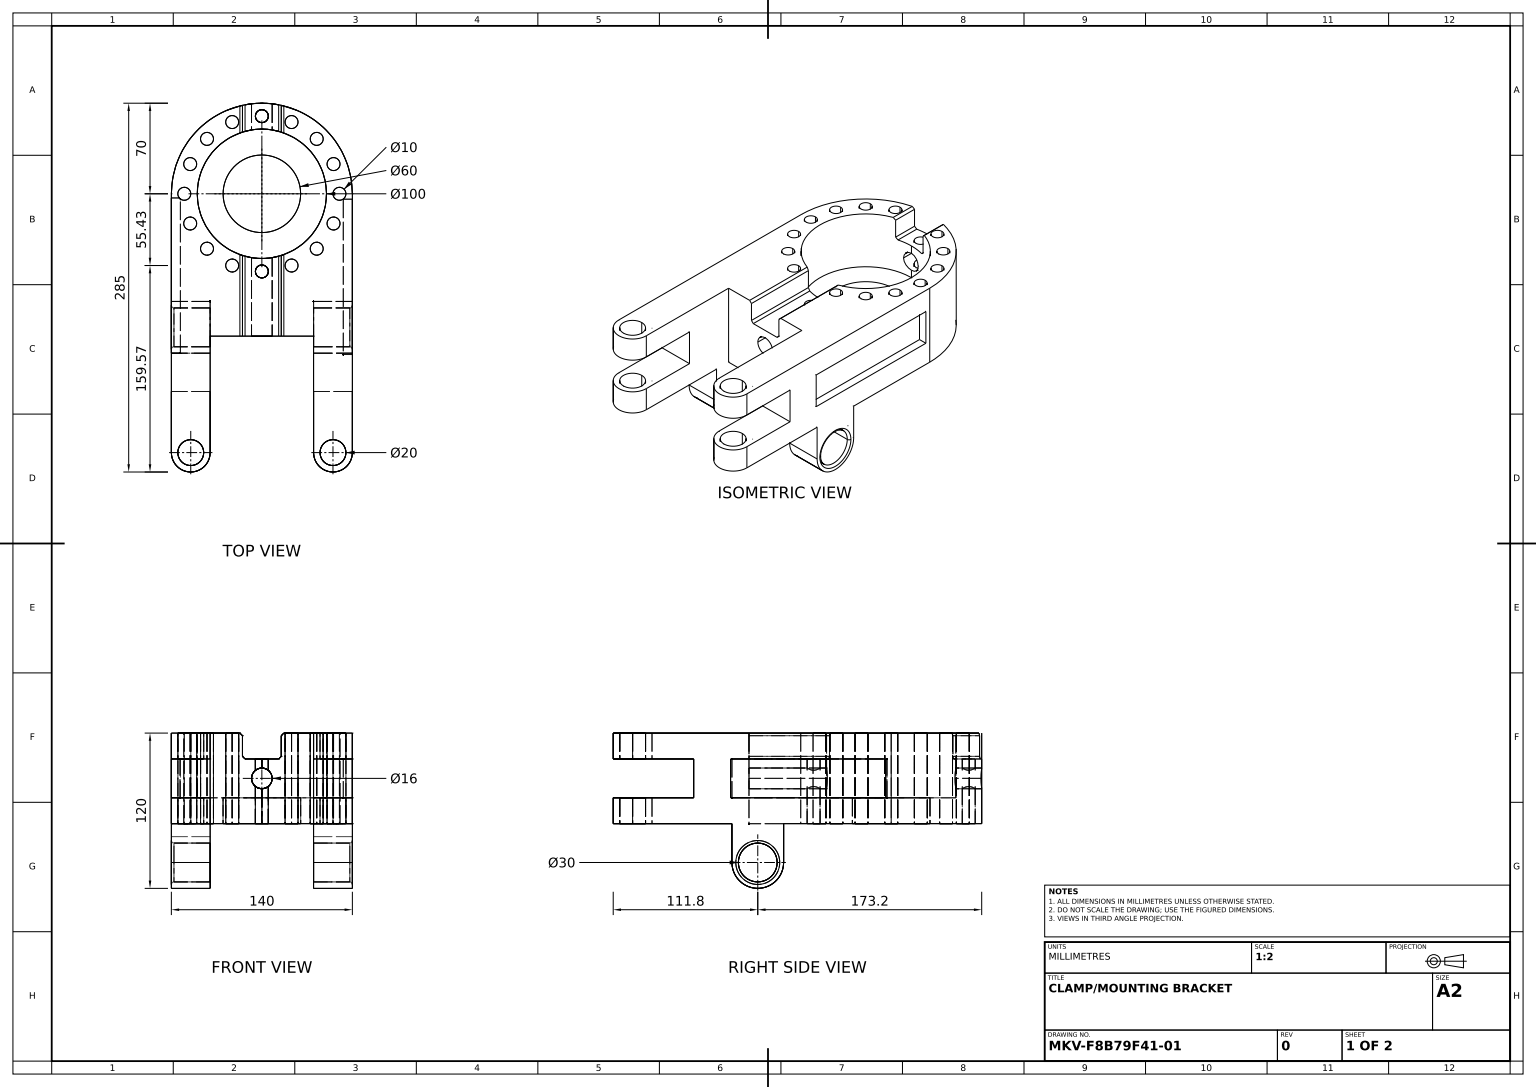
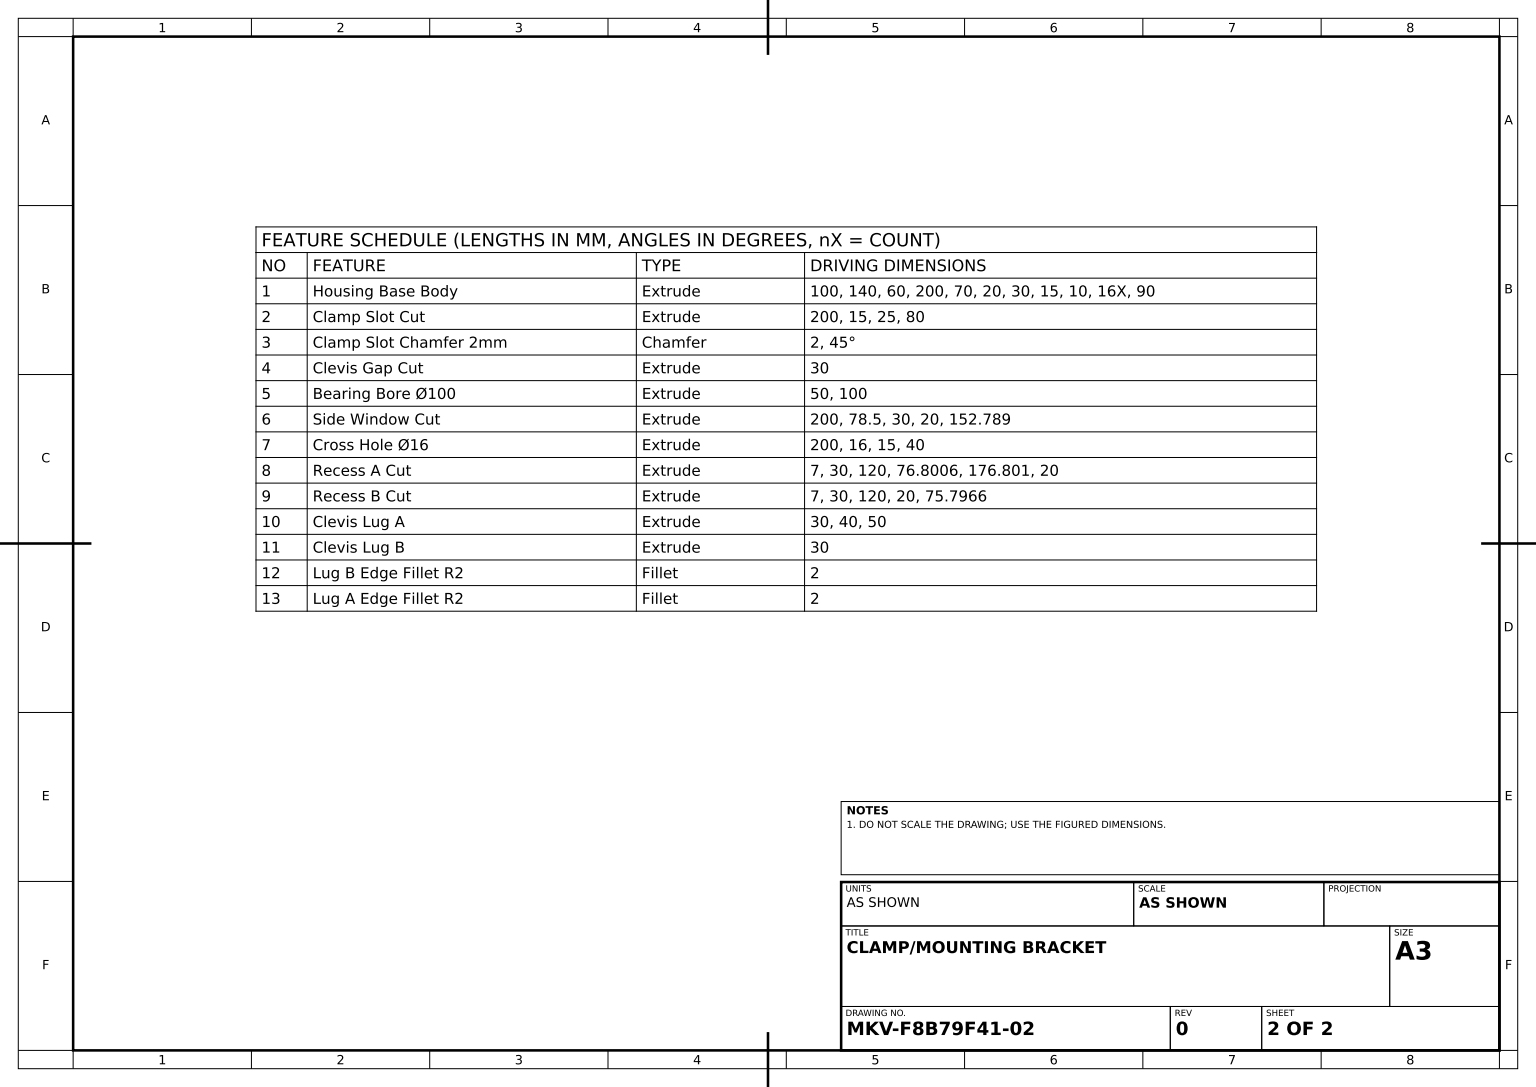
SolidWorks part; units mm, degrees
material "Plain Carbon Steel"
ref_plane "Front Plane" through (0, 0, 0) normal (0, 0, 1) x (1, 0, 0)
ref_plane "Top Plane" through (0, 0, 0) normal (0, 1, 0) x (1, 0, 0)
ref_plane "Right Plane" through (0, 0, 0) normal (1, 0, 0) x (0, 0, -1)
sketch "Housing Base Profile Sketch" plane through (0, 0, 0) normal (0, 1, 0) x (1, 0, 0)
  line L1 (-70, 200) -> (-70, 0)
  line L2 (70, 200) -> (70, 0)
  line L3 (-40, 0) -> (-40, 90)
  line L4 (40, 0) -> (40, 90)
  line L5 (40, 90) -> (-40, 90)
  arc A0 (70, 200) -> (-70, 200) centre (0, 200) ccw
  circle A2 centre (0, 200) radius 30
  circle A3 centre (-55, 0) radius 10
  arc A4 (-70, 0) -> (-40, 0) centre (-55, 0) ccw
  circle A5 centre (55, 0) radius 10
  arc A6 (40, 0) -> (70, 0) centre (55, 0) ccw
  circle A7 centre (0, 260) radius 5
  circle A8 centre (22.961, 255.4328) radius 5
  circle A9 centre (42.4264, 242.4264) radius 5
  circle A10 centre (55.4328, 222.961) radius 5
  circle A11 centre (60, 200) radius 5
  circle A12 centre (55.4328, 177.039) radius 5
  circle A13 centre (42.4264, 157.5736) radius 5
  circle A14 centre (22.961, 144.5672) radius 5
  circle A15 centre (0, 140) radius 5
  circle A16 centre (-22.961, 144.5672) radius 5
  circle A17 centre (-42.4264, 157.5736) radius 5
  circle A18 centre (-55.4328, 177.039) radius 5
  circle A19 centre (-60, 200) radius 5
  circle A20 centre (-55.4328, 222.961) radius 5
  circle A21 centre (-42.4264, 242.4264) radius 5
  circle A22 centre (-22.961, 255.4328) radius 5
  point P8 (0, 0)
  dimension "D1" = 140
  dimension "D2" = 90
  dimension "D3" = 60
  dimension "D6" = 60
  dimension "D7" = 20
  dimension "D8" = 20
  dimension "D9" = 30
  dimension "D12" = 10
  dimension "D4" = 200
  dimension "D5" = 70
  dimension "D11" = 15
  dimension "D13" = 16
extrude "Housing Base Body" add sketch "Housing Base Profile Sketch" along normal blind 100
sketch "Clamp Slot Sketch" plane through (0, 0, -90) normal (0, 0, 1) x (1, 0, 0)
  line L0 (-15, 100) -> (15, 100)
  line L1 (-40, 100) -> (40, 100) construction
  line L2 (40, 100) -> (40, 0) construction
  line L3 (-15, 100) -> (15, 100)
  line L4 (-15, 100) -> (-15, 80)
  line L5 (-15, 80) -> (15, 80)
  line L6 (15, 100) -> (15, 80)
  line L7 (-40, 0) -> (40, 0) construction
  point P5 (0, 100)
  line M4 (40, 100) -> (-40, 100)
  dimension "D1" = 15
  dimension "D2" = 25
  dimension "D3" = 80
extrude "Clamp Slot Cut" cut sketch "Clamp Slot Sketch" against normal blind 200 contours L6 L4 L5 M4
chamfer "Clamp Slot Chamfer 2mm" distance 2 angle 45 6 edges at (15, 100, -247.1774) (15, 80, -247.1774) (15, 80, -132.0096) (15, 100, -132.0096) (-15, 80, -132.0096) (-15, 100, -132.0096)
sketch "Clevis Gap Sketch" plane through (0, 0, 0) normal (0, -1, 0) x (1, 0, 0)
  line L0 (-70, 0) -> (-70, -200)
  line L1 (-40, 0) -> (-40, -90)
  line L2 (-40, -90) -> (40, -90)
  line L3 (40, -90) -> (40, 0)
  line L4 (70, 0) -> (70, -200)
  arc A0 (-70, 0) -> (-40, 0) centre (-55, 0) cw
  arc A1 (40, 0) -> (70, 0) centre (55, 0) cw
  arc A2 (-70, -200) -> (70, -200) centre (0, -200) ccw
extrude "Clevis Gap Cut" cut sketch "Clevis Gap Sketch" against normal blind 30
sketch "Bearing Bore Sketch" plane through (0, 100, 0) normal (0, 1, 0) x (1, 0, 0)
  circle A0 centre (0, 200) radius 50
  dimension "D1" = 100
extrude "Bearing Bore Ø100" cut sketch "Bearing Bore Sketch" against normal blind 50
sketch "Side Window Sketch" plane through (-70, 0, 0) normal (-1, 0, 0) x (0, 0, 1)
  line L0 (-47.2114, 80) -> (-47.2114, 50)
  line L1 (-200, 100) -> (-200, 30) construction
  line L2 (0, 30) -> (-200, 30) construction
  line L4 (-47.2114, 80) -> (31.2886, 80)
  line L5 (-47.2114, 80) -> (-47.2114, 50)
  line L6 (-47.2114, 50) -> (31.2886, 50)
  line L7 (31.2886, 80) -> (31.2886, 50)
  line M6 (0, 30) -> (0, 100)
  dimension "D1" = 78.5
  dimension "D2" = 30
  dimension "D3" = 20
  dimension "D4" = 152.7886
extrude "Side Window Cut" cut sketch "Side Window Sketch" against normal blind 200 contours L0 L6 L4 M6 | L7 L4 L6 M6
sketch "Cross Hole Sketch" plane through (0, 0, -90) normal (0, 0, 1) x (1, 0, 0)
  line L0 (-13, 80) -> (13, 80) construction
  line L1 (-40, 100) -> (-40, 30) construction
  circle A0 centre (0, 65) radius 8
  dimension "D1" = 16
  dimension "D2" = 15
  dimension "D3" = 40
extrude "Cross Hole Ø16" cut sketch "Cross Hole Sketch" against normal blind 200
sketch "Recess A Sketch" plane through (-70, 0, 0) normal (-1, 0, 0) x (0, 0, 1)
  line L0 (-200, 100) -> (0, 100) construction
  line L1 (-76.8006, 80) -> (-176.8006, 80)
  line L2 (-76.8006, 80) -> (-76.8006, 50)
  line L3 (-76.8006, 50) -> (-176.8006, 50)
  line L5 (-76.8006, 80) -> (-196.8006, 80)
  line L6 (-76.8006, 80) -> (-76.8006, 50)
  line L7 (-76.8006, 50) -> (-196.8006, 50)
  line L8 (-196.8006, 80) -> (-196.8006, 50)
  dimension "D1" = 30
  dimension "D2" = 76.8006
  dimension "D3" = 120
  dimension "D4" = 176.8006
  dimension "D5" = 20
extrude "Recess A Cut" cut sketch "Recess A Sketch" against normal blind 7 contours L5 L8 L7 L3 L2 L1
sketch "Recess B Sketch" plane through (70, 0, 0) normal (1, 0, 0) x (0, 0, -1)
  line L0 (0, 100) -> (200, 100) construction
  line L2 (195.7966, 80) -> (195.7966, 50)
  line L5 (195.7966, 80) -> (75.7966, 80)
  line L6 (195.7966, 80) -> (195.7966, 50)
  line L7 (195.7966, 50) -> (75.7966, 50)
  line L8 (75.7966, 80) -> (75.7966, 50)
  dimension "D1" = 30
  dimension "D2" = 120
  dimension "D3" = 20
  dimension "D4" = 75.7966
extrude "Recess B Cut" cut sketch "Recess B Sketch" against normal blind 7 contours L5 L8 L7 L2
sketch "Clevis Lug A Sketch" plane through (-70, 0, 0) normal (-1, 0, 0) x (0, 0, 1)
  line L0 (-76.8006, 50) -> (-76.8006, 0)
  line L1 (-116.8006, 0) -> (-116.8006, 50)
  line L2 (-76.8006, 50) -> (-196, 50) construction
  line L3 (-116.8006, 50) -> (-76.8006, 50)
  arc A0 (-116.8006, 0) -> (-76.8006, 0) centre (-96.8006, 0) ccw
  circle A1 centre (-96.8006, 0) radius 15
  dimension "D1" = 40
  dimension "D2" = 30
  dimension "D3" = 50
  dimension "D4" = 50
extrude "Clevis Lug A" add sketch "Clevis Lug A Sketch" against normal blind 30
sketch "Clevis Lug B Sketch" plane through (70, 0, 0) normal (1, 0, 0) x (0, 0, -1)
  line L0 (76.8006, 30) -> (116.8006, 30)
  line L1 (116.8006, 30) -> (116.8006, 0)
  line L2 (76.8006, 0) -> (76.8006, 30)
  circle A0 centre (96.8006, 0) radius 15
  arc A1 (76.8006, 0) -> (116.8006, 0) centre (96.8006, 0) ccw
  dimension "D2" = 30
extrude "Clevis Lug B" add sketch "Clevis Lug B Sketch" against normal blind 30
fillet "Lug B Edge Fillet R2" radius 2 1 edges at (70, 0, -111.8006)
fillet "Lug A Edge Fillet R2" radius 2 1 edges at (-70, 0, -81.8006)
